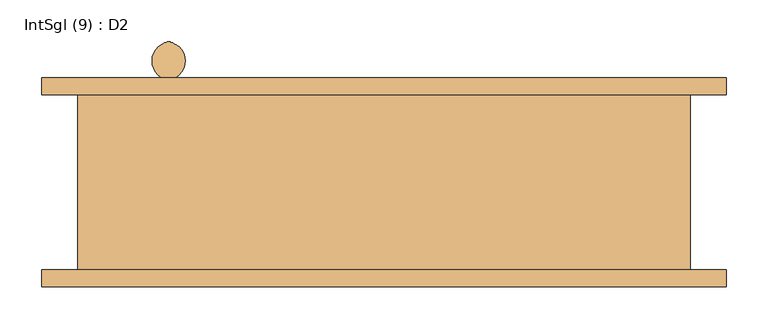
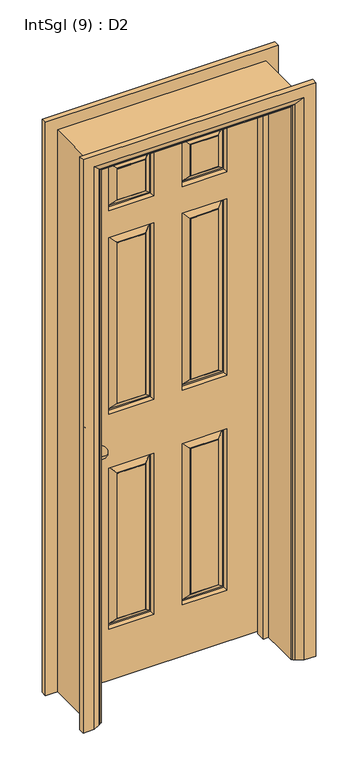
"""IFC4 building model written with IfcOpenShell, lengths in millimetres: door geometry, IntSgl (9) : D2."""

from ifc_helpers import new_model, si_unit, point, frame, origin, place, context, project, spatial, polyline, circle_curve, ellipse_curve, trimmed, outline, extrude, faceted_brep, source, transform, mapped, element, save
from ifc_brep_helpers import plane_surface, cylinder_surface, revolved_surface, advanced_brep


def intsgl_9_d2_d60362bb(model_context):
    return source(origin(), model_context, "Body", "SolidModel", [
        advanced_brep(
        [(-253.0, 48.0, 900.0), (-258.0, 3.562589, 900.0), (-263.0, 48.0, 900.0), (-263.0, 63.0, 900.0), (-253.0, 63.0, 900.0), (-278.0, 67.0, 900.0), (-238.0, 67.0, 900.0), (-278.0, 63.0, 900.0), (-238.0, 63.0, 900.0)],
        [
            (0, 1, circle_curve(frame((-261.1884862, 26.4213505, 900.0), z_axis=(0.0, 0.0, -1.0), x_axis=(0.0, 1.0, 0.0)), 23.0800654)),
            (1, 2, circle_curve(frame((-254.8115138, 26.4213505, 900.0), z_axis=(0.0, 0.0, -1.0), x_axis=(0.0, 1.0, 0.0)), 23.0800654)),
            (2, 0, circle_curve(frame((-258.0, 48.0, 900.0), z_axis=(0.0, -1.0, 0.0), x_axis=(-1.0, 0.0, 0.0)), 5.0)),
            (0, 2, circle_curve(frame((-258.0, 48.0, 900.0), z_axis=(0.0, -1.0, 0.0), x_axis=(-1.0, 0.0, 0.0)), 5.0)),
            (2, 3),
            (3, 4, circle_curve(frame((-258.0, 63.0, 900.0), z_axis=(0.0, -1.0, 0.0), x_axis=(-1.0, 0.0, 0.0)), 5.0)),
            (4, 0),
            (4, 3, circle_curve(frame((-258.0, 63.0, 900.0), z_axis=(0.0, -1.0, 0.0), x_axis=(-1.0, 0.0, 0.0)), 5.0)),
            (5, 6, circle_curve(frame((-258.0, 67.0, 900.0), z_axis=(0.0, 1.0, 0.0), x_axis=(1.0, 0.0, 0.0)), 20.0)),
            (6, 5, circle_curve(frame((-258.0, 67.0, 900.0), z_axis=(0.0, 1.0, 0.0), x_axis=(1.0, 0.0, 0.0)), 20.0)),
            (7, 8, circle_curve(frame((-258.0, 63.0, 900.0), z_axis=(0.0, -1.0, 0.0), x_axis=(1.0, 0.0, 0.0)), 20.0)),
            (8, 7, circle_curve(frame((-258.0, 63.0, 900.0), z_axis=(0.0, -1.0, 0.0), x_axis=(1.0, 0.0, 0.0)), 20.0)),
            (6, 8),
            (7, 5),
        ],
        [
            revolved_surface(trimmed(ellipse_curve(frame((-254.8115138, 26.4213505, 900.0), z_axis=(0.0, 0.0, -1.0), x_axis=(0.0, 1.0, 0.0)), 23.0800654, 23.0800654), [point((-258.0, 3.562589, 900.0))], [point((-263.0, 48.0, 900.0))], True, "CARTESIAN"), (-258.0, 63.0, 900.0), (0.0, 1.0, 0.0)),
            cylinder_surface(frame((-258.0, 63.0, 900.0), z_axis=(0.0, 1.0, 0.0), x_axis=(-1.0, 0.0, 0.0)), 5.0),
            plane_surface(frame((-238.0, 67.0, 900.0), z_axis=(0.0, 1.0, 0.0), x_axis=(0.0, 0.0, 1.0))),
            plane_surface(frame((-238.0, 63.0, 900.0), z_axis=(0.0, -1.0, 0.0), x_axis=(0.0, 0.0, -1.0))),
            cylinder_surface(frame((-258.0, 63.0, 900.0), z_axis=(0.0, 1.0, 0.0), x_axis=(1.0, 0.0, 0.0)), 20.0),
        ],
        [
            (0, [[1, 2, 3]]),
            (0, [[-1, 4, -2]]),
            (1, [[5, 6, 7, -3]]),
            (1, [[-7, 8, -5, -4]]),
            (2, [[9, 10]]),
            (3, [[11, 12], [-8, -6]]),
            (4, [[13, -11, 14, -10]]),
            (4, [[-14, -12, -13, -9]]),
        ],
    ),
        advanced_brep(
        [(-253.0, 124.0, 900.0), (-263.0, 124.0, 900.0), (-258.0, 168.437411, 900.0), (-253.0, 109.0, 900.0), (-263.0, 109.0, 900.0), (-278.0, 105.0, 900.0), (-238.0, 105.0, 900.0), (-278.0, 109.0, 900.0), (-238.0, 109.0, 900.0)],
        [
            (0, 1, circle_curve(frame((-258.0, 124.0, 900.0), z_axis=(0.0, 1.0, 0.0), x_axis=(-1.0, 0.0, 0.0)), 5.0)),
            (1, 2, circle_curve(frame((-254.8115138, 145.5786495, 900.0), z_axis=(0.0, 0.0, -1.0), x_axis=(0.0, -1.0, 0.0)), 23.0800654)),
            (2, 0, circle_curve(frame((-261.1884862, 145.5786495, 900.0), z_axis=(0.0, 0.0, -1.0), x_axis=(0.0, -1.0, 0.0)), 23.0800654)),
            (1, 0, circle_curve(frame((-258.0, 124.0, 900.0), z_axis=(0.0, 1.0, 0.0), x_axis=(-1.0, 0.0, 0.0)), 5.0)),
            (0, 3),
            (3, 4, circle_curve(frame((-258.0, 109.0, 900.0), z_axis=(0.0, 1.0, 0.0), x_axis=(-1.0, 0.0, 0.0)), 5.0)),
            (4, 1),
            (4, 3, circle_curve(frame((-258.0, 109.0, 900.0), z_axis=(0.0, 1.0, 0.0), x_axis=(-1.0, 0.0, 0.0)), 5.0)),
            (5, 6, circle_curve(frame((-258.0, 105.0, 900.0), z_axis=(0.0, -1.0, 0.0), x_axis=(1.0, 0.0, 0.0)), 20.0)),
            (6, 5, circle_curve(frame((-258.0, 105.0, 900.0), z_axis=(0.0, -1.0, 0.0), x_axis=(1.0, 0.0, 0.0)), 20.0)),
            (7, 8, circle_curve(frame((-258.0, 109.0, 900.0), z_axis=(0.0, 1.0, 0.0), x_axis=(1.0, 0.0, 0.0)), 20.0)),
            (8, 7, circle_curve(frame((-258.0, 109.0, 900.0), z_axis=(0.0, 1.0, 0.0), x_axis=(1.0, 0.0, 0.0)), 20.0)),
            (5, 7),
            (8, 6),
        ],
        [
            revolved_surface(trimmed(ellipse_curve(frame((-254.8115138, 145.5786495, 900.0), z_axis=(0.0, 0.0, 1.0), x_axis=(0.0, -1.0, 0.0)), 23.0800654, 23.0800654), [point((-258.0, 168.437411, 900.0))], [point((-263.0, 124.0, 900.0))], True, "CARTESIAN"), (-258.0, 109.0, 900.0), (0.0, -1.0, 0.0)),
            cylinder_surface(frame((-258.0, 109.0, 900.0), z_axis=(0.0, -1.0, 0.0), x_axis=(-1.0, 0.0, 0.0)), 5.0),
            plane_surface(frame((-238.0, 105.0, 900.0), z_axis=(0.0, -1.0, 0.0), x_axis=(0.0, 0.0, 1.0))),
            plane_surface(frame((-238.0, 109.0, 900.0), z_axis=(0.0, 1.0, 0.0), x_axis=(0.0, 0.0, -1.0))),
            cylinder_surface(frame((-258.0, 109.0, 900.0), z_axis=(0.0, -1.0, 0.0), x_axis=(1.0, 0.0, 0.0)), 20.0),
        ],
        [
            (0, [[1, 2, 3]]),
            (0, [[-2, 4, -3]]),
            (1, [[-1, 5, 6, 7]]),
            (1, [[-4, -7, 8, -5]]),
            (2, [[9, 10]]),
            (3, [[11, 12], [-6, -8]]),
            (4, [[-9, 13, -12, 14]]),
            (4, [[-10, -14, -11, -13]]),
        ],
    ),
        faceted_brep([(-333.0, 67.0, 2058.0), (-333.0, 67.0, 8.0), (333.0, 67.0, 8.0), (333.0, 67.0, 2058.0), (-50.0, 67.0, 800.0), (-50.0, 67.0, 200.0), (-208.0, 67.0, 200.0), (-208.0, 67.0, 800.0), (208.0, 67.0, 800.0), (208.0, 67.0, 200.0), (50.0, 67.0, 200.0), (50.0, 67.0, 800.0), (-50.0, 67.0, 1658.0), (-50.0, 67.0, 1000.0), (-208.0, 67.0, 1000.0), (-208.0, 67.0, 1658.0), (208.0, 67.0, 1658.0), (208.0, 67.0, 1000.0), (50.0, 67.0, 1000.0), (50.0, 67.0, 1658.0), (-50.0, 67.0, 1933.0), (-50.0, 67.0, 1758.0), (-208.0, 67.0, 1758.0), (-208.0, 67.0, 1933.0), (208.0, 67.0, 1933.0), (208.0, 67.0, 1758.0), (50.0, 67.0, 1758.0), (50.0, 67.0, 1933.0), (-80.0, 67.0, 230.0), (-80.0, 67.0, 770.0), (-178.0, 67.0, 770.0), (-178.0, 67.0, 230.0), (178.0, 67.0, 230.0), (178.0, 67.0, 770.0), (80.0, 67.0, 770.0), (80.0, 67.0, 230.0), (-80.0, 67.0, 1030.0), (-80.0, 67.0, 1628.0), (-178.0, 67.0, 1628.0), (-178.0, 67.0, 1030.0), (178.0, 67.0, 1030.0), (178.0, 67.0, 1628.0), (80.0, 67.0, 1628.0), (80.0, 67.0, 1030.0), (-80.0, 67.0, 1788.0), (-80.0, 67.0, 1903.0), (-178.0, 67.0, 1903.0), (-178.0, 67.0, 1788.0), (178.0, 67.0, 1788.0), (178.0, 67.0, 1903.0), (80.0, 67.0, 1903.0), (80.0, 67.0, 1788.0), (-333.0, 105.0, 2058.0), (333.0, 105.0, 2058.0), (333.0, 105.0, 8.0), (-333.0, 105.0, 8.0), (50.0, 105.0, 800.0), (50.0, 105.0, 200.0), (208.0, 105.0, 200.0), (208.0, 105.0, 800.0), (-208.0, 105.0, 800.0), (-208.0, 105.0, 200.0), (-50.0, 105.0, 200.0), (-50.0, 105.0, 800.0), (50.0, 105.0, 1658.0), (50.0, 105.0, 1000.0), (208.0, 105.0, 1000.0), (208.0, 105.0, 1658.0), (-208.0, 105.0, 1658.0), (-208.0, 105.0, 1000.0), (-50.0, 105.0, 1000.0), (-50.0, 105.0, 1658.0), (50.0, 105.0, 1933.0), (50.0, 105.0, 1758.0), (208.0, 105.0, 1758.0), (208.0, 105.0, 1933.0), (-208.0, 105.0, 1933.0), (-208.0, 105.0, 1758.0), (-50.0, 105.0, 1758.0), (-50.0, 105.0, 1933.0), (80.0, 105.0, 230.0), (80.0, 105.0, 770.0), (178.0, 105.0, 770.0), (178.0, 105.0, 230.0), (-178.0, 105.0, 230.0), (-178.0, 105.0, 770.0), (-80.0, 105.0, 770.0), (-80.0, 105.0, 230.0), (80.0, 105.0, 1030.0), (80.0, 105.0, 1628.0), (178.0, 105.0, 1628.0), (178.0, 105.0, 1030.0), (-178.0, 105.0, 1030.0), (-178.0, 105.0, 1628.0), (-80.0, 105.0, 1628.0), (-80.0, 105.0, 1030.0), (80.0, 105.0, 1788.0), (80.0, 105.0, 1903.0), (178.0, 105.0, 1903.0), (178.0, 105.0, 1788.0), (-178.0, 105.0, 1788.0), (-178.0, 105.0, 1903.0), (-80.0, 105.0, 1903.0), (-80.0, 105.0, 1788.0), (80.0, 104.0, 230.0), (80.0, 104.0, 770.0), (58.0, 90.0, 208.0), (58.0, 90.0, 792.0), (78.0, 104.0, 772.0), (78.0, 104.0, 228.0), (53.0, 90.0, 797.0), (53.0, 90.0, 203.0), (178.0, 104.0, 770.0), (200.0, 90.0, 792.0), (180.0, 104.0, 772.0), (205.0, 90.0, 797.0), (178.0, 104.0, 230.0), (200.0, 90.0, 208.0), (180.0, 104.0, 228.0), (205.0, 90.0, 203.0), (-178.0, 104.0, 230.0), (-178.0, 104.0, 770.0), (-200.0, 90.0, 208.0), (-200.0, 90.0, 792.0), (-180.0, 104.0, 772.0), (-180.0, 104.0, 228.0), (-205.0, 90.0, 797.0), (-205.0, 90.0, 203.0), (-80.0, 104.0, 770.0), (-58.0, 90.0, 792.0), (-78.0, 104.0, 772.0), (-53.0, 90.0, 797.0), (-80.0, 104.0, 230.0), (-58.0, 90.0, 208.0), (-78.0, 104.0, 228.0), (-53.0, 90.0, 203.0), (80.0, 104.0, 1030.0), (80.0, 104.0, 1628.0), (58.0, 90.0, 1008.0), (58.0, 90.0, 1650.0), (78.0, 104.0, 1630.0), (78.0, 104.0, 1028.0), (53.0, 90.0, 1655.0), (53.0, 90.0, 1003.0), (178.0, 104.0, 1628.0), (200.0, 90.0, 1650.0), (180.0, 104.0, 1630.0), (205.0, 90.0, 1655.0), (178.0, 104.0, 1030.0), (200.0, 90.0, 1008.0), (180.0, 104.0, 1028.0), (205.0, 90.0, 1003.0), (-178.0, 104.0, 1030.0), (-178.0, 104.0, 1628.0), (-200.0, 90.0, 1008.0), (-200.0, 90.0, 1650.0), (-180.0, 104.0, 1630.0), (-180.0, 104.0, 1028.0), (-205.0, 90.0, 1655.0), (-205.0, 90.0, 1003.0), (-80.0, 104.0, 1628.0), (-58.0, 90.0, 1650.0), (-78.0, 104.0, 1630.0), (-53.0, 90.0, 1655.0), (-80.0, 104.0, 1030.0), (-58.0, 90.0, 1008.0), (-78.0, 104.0, 1028.0), (-53.0, 90.0, 1003.0), (80.0, 104.0, 1788.0), (80.0, 104.0, 1903.0), (58.0, 90.0, 1766.0), (58.0, 90.0, 1925.0), (78.0, 104.0, 1905.0), (78.0, 104.0, 1786.0), (53.0, 90.0, 1930.0), (53.0, 90.0, 1761.0), (178.0, 104.0, 1903.0), (200.0, 90.0, 1925.0), (180.0, 104.0, 1905.0), (205.0, 90.0, 1930.0), (178.0, 104.0, 1788.0), (200.0, 90.0, 1766.0), (180.0, 104.0, 1786.0), (205.0, 90.0, 1761.0), (-178.0, 104.0, 1788.0), (-178.0, 104.0, 1903.0), (-200.0, 90.0, 1766.0), (-200.0, 90.0, 1925.0), (-180.0, 104.0, 1905.0), (-180.0, 104.0, 1786.0), (-205.0, 90.0, 1930.0), (-205.0, 90.0, 1761.0), (-80.0, 104.0, 1903.0), (-58.0, 90.0, 1925.0), (-78.0, 104.0, 1905.0), (-53.0, 90.0, 1930.0), (-80.0, 104.0, 1788.0), (-58.0, 90.0, 1766.0), (-78.0, 104.0, 1786.0), (-53.0, 90.0, 1761.0), (-80.0, 68.0, 230.0), (-80.0, 68.0, 770.0), (-58.0, 82.0, 208.0), (-58.0, 82.0, 792.0), (-78.0, 68.0, 772.0), (-78.0, 68.0, 228.0), (-53.0, 82.0, 797.0), (-53.0, 82.0, 203.0), (-178.0, 68.0, 770.0), (-200.0, 82.0, 792.0), (-180.0, 68.0, 772.0), (-205.0, 82.0, 797.0), (-178.0, 68.0, 230.0), (-200.0, 82.0, 208.0), (-180.0, 68.0, 228.0), (-205.0, 82.0, 203.0), (178.0, 68.0, 230.0), (178.0, 68.0, 770.0), (200.0, 82.0, 208.0), (200.0, 82.0, 792.0), (180.0, 68.0, 772.0), (180.0, 68.0, 228.0), (205.0, 82.0, 797.0), (205.0, 82.0, 203.0), (80.0, 68.0, 770.0), (58.0, 82.0, 792.0), (78.0, 68.0, 772.0), (53.0, 82.0, 797.0), (80.0, 68.0, 230.0), (58.0, 82.0, 208.0), (78.0, 68.0, 228.0), (53.0, 82.0, 203.0), (-80.0, 68.0, 1030.0), (-80.0, 68.0, 1628.0), (-58.0, 82.0, 1008.0), (-58.0, 82.0, 1650.0), (-78.0, 68.0, 1630.0), (-78.0, 68.0, 1028.0), (-53.0, 82.0, 1655.0), (-53.0, 82.0, 1003.0), (-178.0, 68.0, 1628.0), (-200.0, 82.0, 1650.0), (-180.0, 68.0, 1630.0), (-205.0, 82.0, 1655.0), (-178.0, 68.0, 1030.0), (-200.0, 82.0, 1008.0), (-180.0, 68.0, 1028.0), (-205.0, 82.0, 1003.0), (178.0, 68.0, 1030.0), (178.0, 68.0, 1628.0), (200.0, 82.0, 1008.0), (200.0, 82.0, 1650.0), (180.0, 68.0, 1630.0), (180.0, 68.0, 1028.0), (205.0, 82.0, 1655.0), (205.0, 82.0, 1003.0), (80.0, 68.0, 1628.0), (58.0, 82.0, 1650.0), (78.0, 68.0, 1630.0), (53.0, 82.0, 1655.0), (80.0, 68.0, 1030.0), (58.0, 82.0, 1008.0), (78.0, 68.0, 1028.0), (53.0, 82.0, 1003.0), (-80.0, 68.0, 1788.0), (-80.0, 68.0, 1903.0), (-58.0, 82.0, 1766.0), (-58.0, 82.0, 1925.0), (-78.0, 68.0, 1905.0), (-78.0, 68.0, 1786.0), (-53.0, 82.0, 1930.0), (-53.0, 82.0, 1761.0), (-178.0, 68.0, 1903.0), (-200.0, 82.0, 1925.0), (-180.0, 68.0, 1905.0), (-205.0, 82.0, 1930.0), (-178.0, 68.0, 1788.0), (-200.0, 82.0, 1766.0), (-180.0, 68.0, 1786.0), (-205.0, 82.0, 1761.0), (178.0, 68.0, 1788.0), (178.0, 68.0, 1903.0), (200.0, 82.0, 1766.0), (200.0, 82.0, 1925.0), (180.0, 68.0, 1905.0), (180.0, 68.0, 1786.0), (205.0, 82.0, 1930.0), (205.0, 82.0, 1761.0), (80.0, 68.0, 1903.0), (58.0, 82.0, 1925.0), (78.0, 68.0, 1905.0), (53.0, 82.0, 1930.0), (80.0, 68.0, 1788.0), (58.0, 82.0, 1766.0), (78.0, 68.0, 1786.0), (53.0, 82.0, 1761.0)], [[[0, 1, 2, 3], [4, 5, 6, 7], [8, 9, 10, 11], [12, 13, 14, 15], [16, 17, 18, 19], [20, 21, 22, 23], [24, 25, 26, 27]], [[28, 29, 30, 31]], [[32, 33, 34, 35]], [[36, 37, 38, 39]], [[40, 41, 42, 43]], [[44, 45, 46, 47]], [[48, 49, 50, 51]], [[52, 53, 54, 55], [56, 57, 58, 59], [60, 61, 62, 63], [64, 65, 66, 67], [68, 69, 70, 71], [72, 73, 74, 75], [76, 77, 78, 79]], [[80, 81, 82, 83]], [[84, 85, 86, 87]], [[88, 89, 90, 91]], [[92, 93, 94, 95]], [[96, 97, 98, 99]], [[100, 101, 102, 103]], [[1, 0, 52, 55]], [[2, 1, 55, 54]], [[3, 2, 54, 53]], [[0, 3, 53, 52]], [[104, 105, 81, 80]], [[106, 107, 108, 109]], [[56, 110, 111, 57]], [[81, 105, 112, 82]], [[108, 107, 113, 114]], [[110, 56, 59, 115]], [[82, 112, 116, 83]], [[114, 113, 117, 118]], [[115, 59, 58, 119]], [[104, 80, 83, 116]], [[109, 108, 114, 118], [105, 104, 116, 112]], [[106, 109, 118, 117]], [[111, 110, 115, 119], [107, 106, 117, 113]], [[57, 111, 119, 58]], [[120, 121, 85, 84]], [[122, 123, 124, 125]], [[60, 126, 127, 61]], [[85, 121, 128, 86]], [[124, 123, 129, 130]], [[126, 60, 63, 131]], [[86, 128, 132, 87]], [[130, 129, 133, 134]], [[131, 63, 62, 135]], [[120, 84, 87, 132]], [[125, 124, 130, 134], [121, 120, 132, 128]], [[122, 125, 134, 133]], [[127, 126, 131, 135], [123, 122, 133, 129]], [[61, 127, 135, 62]], [[136, 137, 89, 88]], [[138, 139, 140, 141]], [[64, 142, 143, 65]], [[89, 137, 144, 90]], [[140, 139, 145, 146]], [[142, 64, 67, 147]], [[90, 144, 148, 91]], [[146, 145, 149, 150]], [[147, 67, 66, 151]], [[136, 88, 91, 148]], [[141, 140, 146, 150], [137, 136, 148, 144]], [[138, 141, 150, 149]], [[143, 142, 147, 151], [139, 138, 149, 145]], [[65, 143, 151, 66]], [[152, 153, 93, 92]], [[154, 155, 156, 157]], [[68, 158, 159, 69]], [[93, 153, 160, 94]], [[156, 155, 161, 162]], [[158, 68, 71, 163]], [[94, 160, 164, 95]], [[162, 161, 165, 166]], [[163, 71, 70, 167]], [[152, 92, 95, 164]], [[157, 156, 162, 166], [153, 152, 164, 160]], [[154, 157, 166, 165]], [[159, 158, 163, 167], [155, 154, 165, 161]], [[69, 159, 167, 70]], [[168, 169, 97, 96]], [[170, 171, 172, 173]], [[72, 174, 175, 73]], [[97, 169, 176, 98]], [[172, 171, 177, 178]], [[174, 72, 75, 179]], [[98, 176, 180, 99]], [[178, 177, 181, 182]], [[179, 75, 74, 183]], [[168, 96, 99, 180]], [[173, 172, 178, 182], [169, 168, 180, 176]], [[170, 173, 182, 181]], [[175, 174, 179, 183], [171, 170, 181, 177]], [[73, 175, 183, 74]], [[184, 185, 101, 100]], [[186, 187, 188, 189]], [[76, 190, 191, 77]], [[101, 185, 192, 102]], [[188, 187, 193, 194]], [[190, 76, 79, 195]], [[102, 192, 196, 103]], [[194, 193, 197, 198]], [[195, 79, 78, 199]], [[184, 100, 103, 196]], [[189, 188, 194, 198], [185, 184, 196, 192]], [[186, 189, 198, 197]], [[191, 190, 195, 199], [187, 186, 197, 193]], [[77, 191, 199, 78]], [[200, 201, 29, 28]], [[202, 203, 204, 205]], [[4, 206, 207, 5]], [[29, 201, 208, 30]], [[204, 203, 209, 210]], [[206, 4, 7, 211]], [[30, 208, 212, 31]], [[210, 209, 213, 214]], [[211, 7, 6, 215]], [[200, 28, 31, 212]], [[205, 204, 210, 214], [201, 200, 212, 208]], [[202, 205, 214, 213]], [[207, 206, 211, 215], [203, 202, 213, 209]], [[5, 207, 215, 6]], [[216, 217, 33, 32]], [[218, 219, 220, 221]], [[8, 222, 223, 9]], [[33, 217, 224, 34]], [[220, 219, 225, 226]], [[222, 8, 11, 227]], [[34, 224, 228, 35]], [[226, 225, 229, 230]], [[227, 11, 10, 231]], [[216, 32, 35, 228]], [[221, 220, 226, 230], [217, 216, 228, 224]], [[218, 221, 230, 229]], [[223, 222, 227, 231], [219, 218, 229, 225]], [[9, 223, 231, 10]], [[232, 233, 37, 36]], [[234, 235, 236, 237]], [[12, 238, 239, 13]], [[37, 233, 240, 38]], [[236, 235, 241, 242]], [[238, 12, 15, 243]], [[38, 240, 244, 39]], [[242, 241, 245, 246]], [[243, 15, 14, 247]], [[232, 36, 39, 244]], [[237, 236, 242, 246], [233, 232, 244, 240]], [[234, 237, 246, 245]], [[239, 238, 243, 247], [235, 234, 245, 241]], [[13, 239, 247, 14]], [[248, 249, 41, 40]], [[250, 251, 252, 253]], [[16, 254, 255, 17]], [[41, 249, 256, 42]], [[252, 251, 257, 258]], [[254, 16, 19, 259]], [[42, 256, 260, 43]], [[258, 257, 261, 262]], [[259, 19, 18, 263]], [[248, 40, 43, 260]], [[253, 252, 258, 262], [249, 248, 260, 256]], [[250, 253, 262, 261]], [[255, 254, 259, 263], [251, 250, 261, 257]], [[17, 255, 263, 18]], [[264, 265, 45, 44]], [[266, 267, 268, 269]], [[20, 270, 271, 21]], [[45, 265, 272, 46]], [[268, 267, 273, 274]], [[270, 20, 23, 275]], [[46, 272, 276, 47]], [[274, 273, 277, 278]], [[275, 23, 22, 279]], [[264, 44, 47, 276]], [[269, 268, 274, 278], [265, 264, 276, 272]], [[266, 269, 278, 277]], [[271, 270, 275, 279], [267, 266, 277, 273]], [[21, 271, 279, 22]], [[280, 281, 49, 48]], [[282, 283, 284, 285]], [[24, 286, 287, 25]], [[49, 281, 288, 50]], [[284, 283, 289, 290]], [[286, 24, 27, 291]], [[50, 288, 292, 51]], [[290, 289, 293, 294]], [[291, 27, 26, 295]], [[280, 48, 51, 292]], [[285, 284, 290, 294], [281, 280, 292, 288]], [[282, 285, 294, 293]], [[287, 286, 291, 295], [283, 282, 293, 289]], [[25, 287, 295, 26]]]),
        faceted_brep([(-335.0, 105.0, 0.0), (-335.0, -105.0, 0.0), (-367.0, -105.0, 0.0), (-367.0, 105.0, 0.0), (-335.0, 105.0, 2060.0), (-335.0, -105.0, 2060.0), (-367.0, -105.0, 2092.0), (-367.0, 105.0, 2092.0), (335.0, 105.0, 0.0), (367.0, 105.0, 0.0), (367.0, -105.0, 0.0), (335.0, -105.0, 0.0), (335.0, 105.0, 2060.0), (367.0, 105.0, 2092.0), (367.0, -105.0, 2092.0), (335.0, -105.0, 2060.0)], [[[0, 1, 2, 3]], [[1, 0, 4, 5]], [[2, 1, 5, 6]], [[3, 2, 6, 7]], [[0, 3, 7, 4]], [[8, 9, 10, 11]], [[12, 13, 9, 8]], [[13, 14, 10, 9]], [[14, 15, 11, 10]], [[15, 12, 8, 11]], [[5, 4, 12, 15]], [[6, 5, 15, 14]], [[7, 6, 14, 13]], [[4, 7, 13, 12]]]),
        extrude(outline(polyline([(0.0, -335.0), (0.0, -316.0), (2041.0, -316.0), (2041.0, 316.0), (0.0, 316.0), (0.0, 335.0), (2060.0, 335.0), (2060.0, -335.0), (0.0, -335.0)])), frame((0.0, 33.0, 0.0), z_axis=(0.0, 1.0, 0.0), x_axis=(0.0, 0.0, 1.0)), (0.0, 0.0, 1.0), 32.0),
        advanced_brep(
        [(-410.0, -125.0, 0.0), (-410.0, -105.0, 0.0), (-340.0, -105.0, 0.0), (-344.0, -111.0, 0.0), (-370.0, -125.0, 0.0), (-410.0, -125.0, 2135.0), (-410.0, -105.0, 2135.0), (410.0, -105.0, 2135.0), (410.0, -105.0, 0.0), (340.0, -105.0, 0.0), (340.0, -105.0, 2065.0), (-340.0, -105.0, 2065.0), (-344.0, -111.0, 2069.0), (-370.0, -125.0, 2095.0), (370.0, -125.0, 2095.0), (370.0, -125.0, 0.0), (410.0, -125.0, 0.0), (410.0, -125.0, 2135.0), (344.0, -111.0, 0.0), (344.0, -111.0, 2069.0)],
        [
            (0, 1),
            (1, 2),
            (2, 3, circle_curve(frame((-348.0, -104.0, 0.0), z_axis=(0.0, 0.0, -1.0), x_axis=(-1.0, 0.0, 0.0)), 8.0622577)),
            (3, 4),
            (4, 0),
            (0, 5),
            (5, 6),
            (6, 1),
            (6, 7),
            (7, 8),
            (8, 9),
            (9, 10),
            (10, 11),
            (11, 2),
            (11, 12, ellipse_curve(frame((-348.0, -104.0, 2073.0), z_axis=(-0.7071067811865475, 0.0, -0.7071067811865475), x_axis=(0.7071067811865474, 0.0, -0.7071067811865476)), 11.4017543, 8.0622577)),
            (12, 3),
            (12, 13),
            (13, 4),
            (13, 14),
            (14, 15),
            (15, 16),
            (16, 17),
            (17, 5),
            (7, 17),
            (16, 8),
            (15, 18),
            (18, 9, circle_curve(frame((348.0, -104.0, 0.0), z_axis=(0.0, 0.0, -1.0), x_axis=(1.0, 0.0, 0.0)), 8.0622577)),
            (19, 10, ellipse_curve(frame((348.0, -104.0, 2073.0), z_axis=(0.7071067811865475, 0.0, -0.7071067811865475), x_axis=(0.7071067811865474, 0.0, 0.7071067811865476)), 11.4017543, 8.0622577)),
            (18, 19),
            (14, 19),
            (19, 12),
        ],
        [
            plane_surface(frame((-340.0, -105.0, 0.0), z_axis=(0.0, 0.0, -1.0), x_axis=(0.0, -1.0, 0.0))),
            plane_surface(frame((-410.0, -125.0, 0.0), z_axis=(-1.0, 0.0, 0.0), x_axis=(0.0, 0.0, 1.0))),
            plane_surface(frame((-410.0, -105.0, 0.0), z_axis=(0.0, 1.0, 0.0), x_axis=(0.0, 0.0, 1.0))),
            cylinder_surface(frame((-348.0, -104.0, 0.0), z_axis=(0.0, 0.0, -1.0), x_axis=(-1.0, 0.0, 0.0)), 8.0622577),
            plane_surface(frame((-344.0, -111.0, 0.0), z_axis=(0.4740998230350183, -0.8804710999221749, 0.0), x_axis=(0.0, 0.0, 1.0))),
            plane_surface(frame((-370.0, -125.0, 0.0), z_axis=(0.0, -1.0, 0.0), x_axis=(0.0, 0.0, 1.0))),
            plane_surface(frame((410.0, -125.0, 2135.0), z_axis=(1.0, 0.0, 0.0), x_axis=(0.0, 0.0, -1.0))),
            plane_surface(frame((340.0, -105.0, 0.0), z_axis=(0.0, 0.0, -1.0), x_axis=(0.0, -1.0, 0.0))),
            cylinder_surface(frame((348.0, -104.0, 2065.0), z_axis=(0.0, 0.0, 1.0), x_axis=(1.0, 0.0, 0.0)), 8.0622577),
            plane_surface(frame((344.0, -111.0, 2069.0), z_axis=(-0.4740998230350183, -0.8804710999221749, 0.0), x_axis=(0.0, 0.0, -1.0))),
            plane_surface(frame((-410.0, -125.0, 2135.0), z_axis=(0.0, 0.0, 1.0), x_axis=(1.0, 0.0, 0.0))),
            cylinder_surface(frame((-340.0, -104.0, 2073.0), z_axis=(-1.0, 0.0, 0.0), x_axis=(0.0, 0.0, 1.0)), 8.0622577),
            plane_surface(frame((-344.0, -111.0, 2069.0), z_axis=(0.0, -0.8804710999221749, -0.4740998230350183), x_axis=(1.0, 0.0, 0.0))),
        ],
        [
            (0, [[1, 2, 3, 4, 5]]),
            (1, [[-1, 6, 7, 8]]),
            (2, [[-2, -8, 9, 10, 11, 12, 13, 14]]),
            (3, [[-3, -14, 15, 16]]),
            (4, [[-4, -16, 17, 18]]),
            (5, [[-5, -18, 19, 20, 21, 22, 23, -6]]),
            (6, [[24, -22, 25, -10]]),
            (7, [[-21, 26, 27, -11, -25]]),
            (8, [[28, -12, -27, 29]]),
            (9, [[30, -29, -26, -20]]),
            (10, [[-7, -23, -24, -9]]),
            (11, [[-15, -13, -28, 31]]),
            (12, [[-17, -31, -30, -19]]),
        ],
    ),
        advanced_brep(
        [(410.0, 125.0, 0.0), (410.0, 105.0, 0.0), (340.0, 105.0, 0.0), (344.0, 111.0, 0.0), (370.0, 125.0, 0.0), (410.0, 125.0, 2135.0), (410.0, 105.0, 2135.0), (-410.0, 105.0, 2135.0), (-410.0, 105.0, 0.0), (-340.0, 105.0, 0.0), (-340.0, 105.0, 2065.0), (340.0, 105.0, 2065.0), (344.0, 111.0, 2069.0), (370.0, 125.0, 2095.0), (-370.0, 125.0, 2095.0), (-370.0, 125.0, 0.0), (-410.0, 125.0, 0.0), (-410.0, 125.0, 2135.0), (-344.0, 111.0, 0.0), (-344.0, 111.0, 2069.0)],
        [
            (0, 1),
            (1, 2),
            (2, 3, circle_curve(frame((348.0, 104.0, 0.0), z_axis=(0.0, 0.0, -1.0), x_axis=(1.0, 0.0, 0.0)), 8.0622577)),
            (3, 4),
            (4, 0),
            (0, 5),
            (5, 6),
            (6, 1),
            (6, 7),
            (7, 8),
            (8, 9),
            (9, 10),
            (10, 11),
            (11, 2),
            (11, 12, ellipse_curve(frame((348.0, 104.0, 2073.0), z_axis=(0.7071067811865475, 0.0, -0.7071067811865475), x_axis=(-0.7071067811865474, 0.0, -0.7071067811865476)), 11.4017543, 8.0622577)),
            (12, 3),
            (12, 13),
            (13, 4),
            (13, 14),
            (14, 15),
            (15, 16),
            (16, 17),
            (17, 5),
            (7, 17),
            (16, 8),
            (15, 18),
            (18, 9, circle_curve(frame((-348.0, 104.0, 0.0), z_axis=(0.0, 0.0, -1.0), x_axis=(-1.0, 0.0, 0.0)), 8.0622577)),
            (19, 10, ellipse_curve(frame((-348.0, 104.0, 2073.0), z_axis=(-0.7071067811865475, 0.0, -0.7071067811865475), x_axis=(-0.7071067811865474, 0.0, 0.7071067811865476)), 11.4017543, 8.0622577)),
            (18, 19),
            (14, 19),
            (19, 12),
        ],
        [
            plane_surface(frame((340.0, 105.0, 0.0), z_axis=(0.0, 0.0, -1.0), x_axis=(0.0, 1.0, 0.0))),
            plane_surface(frame((410.0, 125.0, 0.0), z_axis=(1.0, 0.0, 0.0), x_axis=(0.0, 0.0, 1.0))),
            plane_surface(frame((410.0, 105.0, 0.0), z_axis=(0.0, -1.0, 0.0), x_axis=(0.0, 0.0, 1.0))),
            cylinder_surface(frame((348.0, 104.0, 0.0), z_axis=(0.0, 0.0, -1.0), x_axis=(1.0, 0.0, 0.0)), 8.0622577),
            plane_surface(frame((344.0, 111.0, 0.0), z_axis=(-0.4740998230350183, 0.8804710999221749, 0.0), x_axis=(0.0, 0.0, 1.0))),
            plane_surface(frame((370.0, 125.0, 0.0), z_axis=(0.0, 1.0, 0.0), x_axis=(0.0, 0.0, 1.0))),
            plane_surface(frame((-410.0, 125.0, 2135.0), z_axis=(-1.0, 0.0, 0.0), x_axis=(0.0, 0.0, -1.0))),
            plane_surface(frame((-340.0, 105.0, 0.0), z_axis=(0.0, 0.0, -1.0), x_axis=(0.0, 1.0, 0.0))),
            cylinder_surface(frame((-348.0, 104.0, 2065.0), z_axis=(0.0, 0.0, 1.0), x_axis=(-1.0, 0.0, 0.0)), 8.0622577),
            plane_surface(frame((-344.0, 111.0, 2069.0), z_axis=(0.4740998230350183, 0.8804710999221749, 0.0), x_axis=(0.0, 0.0, -1.0))),
            plane_surface(frame((410.0, 125.0, 2135.0), z_axis=(0.0, 0.0, 1.0), x_axis=(-1.0, 0.0, 0.0))),
            cylinder_surface(frame((340.0, 104.0, 2073.0), z_axis=(1.0, 0.0, 0.0), x_axis=(0.0, 0.0, 1.0)), 8.0622577),
            plane_surface(frame((344.0, 111.0, 2069.0), z_axis=(0.0, 0.8804710999221749, -0.4740998230350183), x_axis=(-1.0, 0.0, 0.0))),
        ],
        [
            (0, [[1, 2, 3, 4, 5]]),
            (1, [[-1, 6, 7, 8]]),
            (2, [[-2, -8, 9, 10, 11, 12, 13, 14]]),
            (3, [[-3, -14, 15, 16]]),
            (4, [[-4, -16, 17, 18]]),
            (5, [[-5, -18, 19, 20, 21, 22, 23, -6]]),
            (6, [[24, -22, 25, -10]]),
            (7, [[-21, 26, 27, -11, -25]]),
            (8, [[28, -12, -27, 29]]),
            (9, [[30, -29, -26, -20]]),
            (10, [[-7, -23, -24, -9]]),
            (11, [[-15, -13, -28, 31]]),
            (12, [[-17, -31, -30, -19]]),
        ],
    ),
    ])


if __name__ == "__main__":
    model = new_model("IFC4")
    model_context = context("Model", 3, world=origin())
    ifc_project = project(units=[si_unit("LENGTHUNIT", "METRE", prefix="MILLI")], contexts=[model_context])
    site = spatial("IfcSite", under=ifc_project)
    building = spatial("IfcBuilding", under=site)
    placement = place(None, origin())
    intsgl_9_d2_shape = intsgl_9_d2_d60362bb(model_context)
    element("IfcDoor", 1, ObjectType="IntSgl (9) : D2", at=placement, inside=building, context=model_context, shape_type="MappedRepresentation", body=[
        mapped(intsgl_9_d2_shape, transform((0.0, 0.0, 0.0), x_axis=(1.0, 0.0, 0.0), y_axis=(0.0, 1.0, 0.0), z_axis=(0.0, 0.0, 1.0))),
    ])
    save(model, "model.ifc")

# Revit data of these elements
# Type "IntSgl (9) : D2"
#   Type Mark = "50"
#   Operation = "SingleSwingRight"
#   Manufacturer = "Revit"
#   Keynote = "L20"
#   UnderCut = 8 mm
#   Tolerance = 2 mm
#   Thickness = 38 mm
#   Structural Tolerance = 8 mm
#   StopDepth = 32 mm
#   Stop Thickness = 19 mm
#   Stile Top Rail = 125 mm
#   Stile Shutting = 125 mm
#   Stile Muntin Rail = 100 mm
#   Stile Lock Rail = 200 mm
#   Stile Intermediate/Frieze = 100 mm
#   Stile Hanging = 125 mm
#   Stile Bottom Rail = 200 mm
#   Rough Width = 750 mm
#   Rough Height = 2100 mm
#   Height to Top Lock Rail = 1000 mm
#   Handle Z Distance = 900 mm
#   Handle X Distance = 75 mm
#   Frame Thickness = 32 mm
#   Door Panel Width = 666 mm
#   Height = 2100 mm
#   Width = 750 mm
#   Door Panel Thickness = 38 mm
#   Door Panel Offset = 0 mm
#   Door Panel Height = 2050 mm
#   Architrave Setback = 5 mm
#   Vis - Ironmongery = yes
#   Material Ironmongery = Door - Handle
#   Material Frame = Door - Frame/Mullion
#   Material Door = Door - Panel
#   Material Architrave = Door - Architrave
#   Function = (empty or 0)
#   Wall Closure = (empty or 0)
# Element 1 (IfcDoor, "IntSgl (9) : D2")
#   Materials on its faces: "Door - Panel", "Door - Architrave", "Door - Frame/Mullion", "Door - Handle"
# Materials
#   "Door - Handle": colour RGB 0 0 0, transparency 0, Keynote = "P21", Cost = 0, Export to IFC = 0
#   "Door - Frame/Mullion": class "Wood", colour RGB 212 179 113, transparency 0, Keynote = "L20", Cost = 0, Export to IFC = 0
#   "Door - Panel": class "Wood", colour RGB 210 159 95, transparency 0, Keynote = "L20", Cost = 0, Export to IFC = 0
#   "Door - Architrave": class "Wood", colour RGB 154 90 5, transparency 0, Keynote = "P20", Cost = 0, Export to IFC = 0
